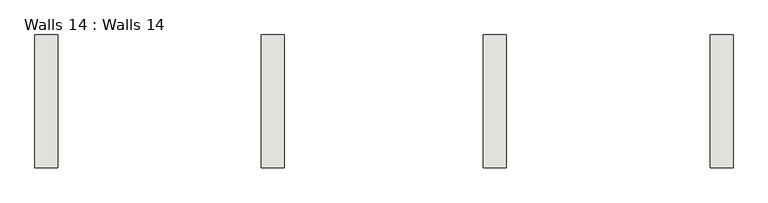
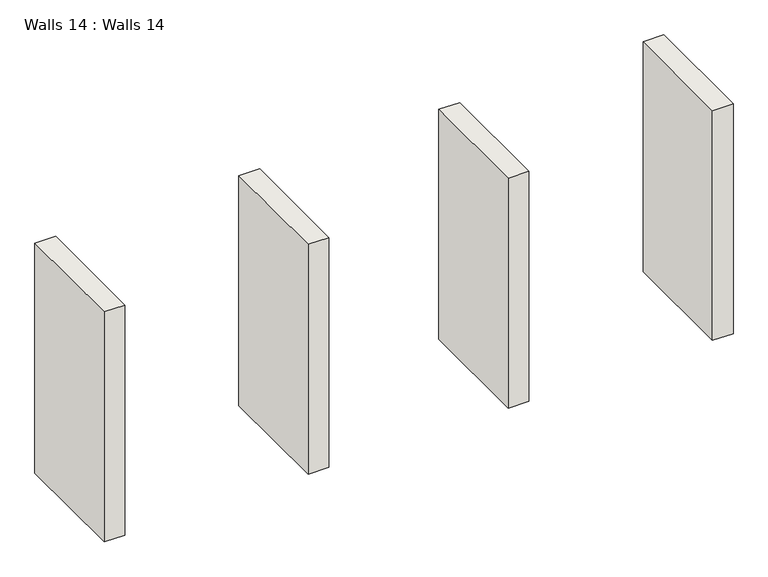
"""IFC4 building model written with IfcOpenShell, lengths in millimetres: wall geometry, Walls 14 : Walls 14."""

from ifc_helpers import new_model, si_unit, frame, origin, place, context, project, spatial, polyline, outline, extrude, source, transform, mapped, element, save


def walls_14_walls_14_a3be32cb(model_context):
    return source(origin(), model_context, "Body", "SweptSolid", [
        extrude(outline(polyline([(-12636.5288845, -2583.4259649), (-12504.8139792, -2583.4259649), (-12504.8139792, -3344.4953156), (-12636.5288845, -3344.4953156), (-12636.5288845, -2583.4259649)])), frame((0.0, 0.0, 1828.8), z_axis=(0.0, 0.0, 1.0), x_axis=(1.0, 0.0, 0.0)), (0.0, 0.0, 1.0), 1543.05),
        extrude(outline(polyline([(-11341.1288845, -2583.4259649), (-11209.4139792, -2583.4259649), (-11209.4139792, -3344.4953156), (-11341.1288845, -3344.4953156), (-11341.1288845, -2583.4259649)])), frame((0.0, 0.0, 1828.8), z_axis=(0.0, 0.0, 1.0), x_axis=(1.0, 0.0, 0.0)), (0.0, 0.0, 1.0), 1543.05),
        extrude(outline(polyline([(-10071.9728698, -2583.4259649), (-9940.2579645, -2583.4259649), (-9940.2579645, -3344.4953156), (-10071.9728698, -3344.4953156), (-10071.9728698, -2583.4259649)])), frame((0.0, 0.0, 1828.8), z_axis=(0.0, 0.0, 1.0), x_axis=(1.0, 0.0, 0.0)), (0.0, 0.0, 1.0), 1543.05),
        extrude(outline(polyline([(-8775.7288845, -2583.4259649), (-8644.0139792, -2583.4259649), (-8644.0139792, -3344.4953156), (-8775.7288845, -3344.4953156), (-8775.7288845, -2583.4259649)])), frame((0.0, 0.0, 1828.8), z_axis=(0.0, 0.0, 1.0), x_axis=(1.0, 0.0, 0.0)), (0.0, 0.0, 1.0), 1543.05),
    ])


if __name__ == "__main__":
    model = new_model("IFC4")
    model_context = context("Model", 3, world=origin())
    ifc_project = project(units=[si_unit("LENGTHUNIT", "METRE", prefix="MILLI")], contexts=[model_context])
    site = spatial("IfcSite", under=ifc_project)
    building = spatial("IfcBuilding", under=site)
    placement = place(None, origin())
    walls_14_walls_14_shape = walls_14_walls_14_a3be32cb(model_context)
    element("IfcWall", 1, ObjectType="Walls 14 : Walls 14", at=placement, inside=building, context=model_context, shape_type="MappedRepresentation", body=[
        mapped(walls_14_walls_14_shape, transform((0.0, 0.0, 0.0), x_axis=(1.0, 0.0, 0.0), y_axis=(0.0, 1.0, 0.0), z_axis=(0.0, 0.0, 1.0))),
    ])
    save(model, "model.ifc")

# Revit data of these elements
# Element 1 (IfcWall, "Walls 14 : Walls 14")
#   Materials on its faces: "Brick, Common"
# Materials
#   "Brick, Common": class "Masonry", colour RGB 0 0 0, transparency 0, Description = "Common brick", Cost = 0
